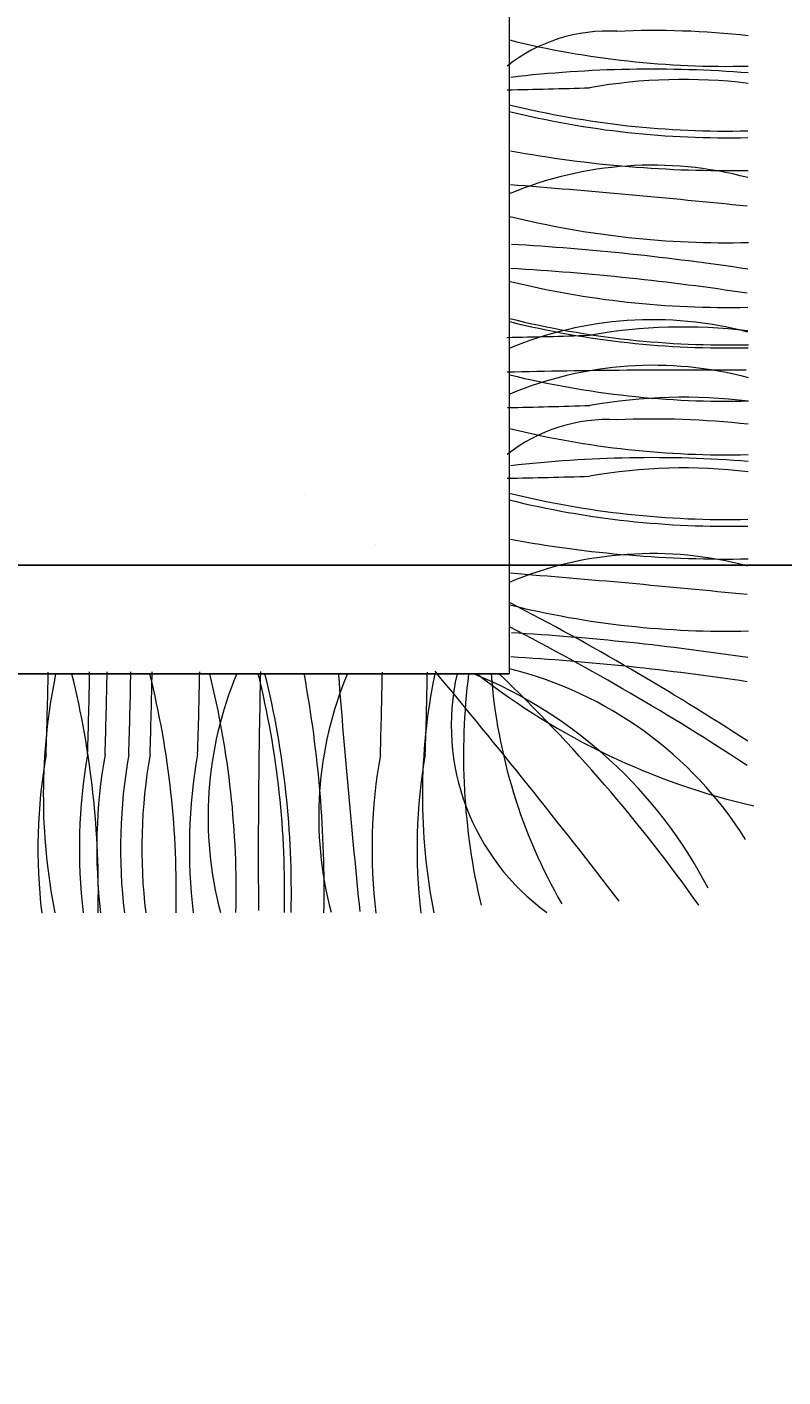
# Model space of a CAD drawing. Units: inches. Extents: x 182 to 1022, y -617 to 111.
# Tile 11 of 33: x 381 to 399, y -308 to -276. Entities that reach past the tile are written whole.
import ezdxf

# ---------------------------------------------------------------- set-up
doc = ezdxf.new("R2010")
doc.units = ezdxf.units.IN
doc.header["$MEASUREMENT"] = 0
doc.layers.add('A-ANNO-DIMS', color=2, linetype='Continuous', lineweight=18)
doc.layers.add('furniture', color=50, linetype='Continuous', lineweight=15, transparency=0.8)
doc.styles.get("Standard").update_dxf_attribs({"font": 'arial.ttf'})
doc.dimstyles.get("Standard").update_dxf_attribs({"dimtxt": 0.18, "dimasz": 0.18, "dimexe": 0.18, "dimexo": 0.0625, "dimgap": 0.09, "dimtad": 0, "dimtih": 1, "dimtoh": 1, "dimdec": 1, "dimzin": 0, "dimdsep": 46, "dimlunit": 4, "dimtxsty": 'Standard', "dimcen": 0.09, "dimadec": 0, "dimazin": 0, "dimtfac": 1, "dimtdec": 1, "dimtofl": 0, "dimtmove": 0, "dimatfit": 3, "dimfxl": 1, "dimtolj": 1, "dimtzin": 0, "dimarcsym": 0})

# ---------------------------------------------------------------- blocks, each defined once
blk = doc.blocks.new('LOUNGE-SEATING-GROUP')
for p, q in [((134.145, 31.682), (134.145, 5.694)), ((137.17, 14.194), (137.17, 14.194)), ((137.705, 14.15), (137.705, 14.15)), ((129.27, 9.969), (129.27, 9.969)), ((130.964, 8.763), (130.964, 8.763)), ((134.145, 5.694), (21.664, 5.694)), ((39.442, 5.694), (134.145, 5.694)), ((130.995, 4.253), (130.995, 4.253)), ((130.995, 4.253), (130.995, 4.253)), ((130.995, 4.253), (130.995, 4.253)), ((132.356, 3.919), (132.356, 3.919)), ((132.356, 3.919), (132.356, 3.919)), ((132.356, 3.919), (132.356, 3.919))]:
    blk.add_line(p, q)
for centre, radius, start, end in [((136.489, 17.128), 3.854, 86.8256, 128.3436), ((137.592, 1.053), 19.942, 83.5587, 92.5565), ((139.313, 41.697), 21.554, 256.1427, 271.3669), ((137.543, -9.04), 29.116, 85.4936, 96.6298), ((131.547, 162.277), 142.714, 271.02248, 271.81091), ((138.293, 7.037), 12.794, 83.1171, 100.0651), ((139.308, 40.158), 21.554, 256.1427, 271.3669), ((139.307, 39.998), 21.554, 256.1427, 271.3669), ((139.339, 46.284), 28.62, 259.5961, 270.9805), ((137.55, 8.956), 8.837, 75.1387, 112.6902), ((114.367, -233.49), 251.596, 84.19829, 85.48538), ((139.318, 37.501), 21.554, 256.1427, 271.3669), ((130.58, -45.595), 61.61, 81.37714, 86.63558), ((130.566, -46.168), 61.61, 81.37714, 86.63558), ((139.301, 35.962), 21.554, 256.1427, 271.3669), ((139.321, 35.071), 21.554, 256.1427, 271.3669), ((137.554, 5.279), 8.837, 75.1387, 112.6902), ((139.309, 34.999), 21.554, 256.1427, 271.3669), ((138.287, 1.148), 12.794, 83.1171, 100.0651), ((131.541, 156.388), 142.714, 271.02248, 271.81091), ((138.51, -171.601), 184.521, 89.60659, 91.37204), ((137.568, 4.195), 8.837, 75.1387, 112.6902), ((139.323, 33.732), 21.554, 256.1427, 271.3669), ((138.299, -0.521), 12.794, 83.1171, 100.0651), ((131.553, 154.719), 142.714, 271.02248, 271.81091), ((136.489, 7.888), 3.854, 86.8256, 128.3436), ((137.592, -8.187), 19.942, 83.5587, 92.5565), ((139.313, 32.457), 21.554, 256.1427, 271.3669), ((137.543, -18.28), 29.116, 85.4936, 96.6298), ((131.547, 153.037), 142.714, 271.02248, 271.81091), ((138.293, -2.203), 12.794, 83.1171, 100.0651), ((139.308, 30.919), 21.554, 256.1427, 271.3669), ((139.307, 30.758), 21.554, 256.1427, 271.3669), ((139.339, 37.044), 28.62, 259.5961, 270.9805), ((137.55, -0.283), 8.837, 75.1387, 112.6902), ((114.367, -242.73), 251.596, 84.19829, 85.48538), ((139.318, 28.261), 21.554, 256.1427, 271.3669), ((105.102, -49.004), 63.435, 56.82194, 62.73315), ((105.088, -49.577), 63.435, 56.82194, 62.73315), ((130.58, -54.835), 61.61, 81.37714, 86.63558), ((131.901, -3.21), 9.302, 32.2712, 76.0065), ((130.566, -55.408), 61.61, 81.37714, 86.63558), ((137.395, 2.803), 14.333, 168.4112, 191.2455), ((-19.513, 8.282), 142.714, 358.18909, 358.97752), ((102.817, 0.521), 21.554, 358.6331, 13.8573), ((-18.527, 8.285), 142.714, 358.18909, 358.97752), ((-18.112, 8.286), 142.714, 358.18909, 358.97752), ((-17.547, 8.287), 142.714, 358.18909, 358.97752), ((104.671, 0.526), 21.554, 358.6331, 13.8573), ((-17.041, 8.289), 142.714, 358.18909, 358.97752), ((-15.91, 8.292), 142.714, 358.18909, 358.97752), ((135.817, 2.285), 8.837, 157.3098, 194.8613), ((106.096, 0.53), 21.554, 358.6331, 13.8573), ((107.248, 0.531), 21.554, 358.6331, 13.8573), ((312.696, 1.329), 184.521, 178.62796, 180.39341), ((107.408, 0.532), 21.554, 358.6331, 13.8573), ((101.122, 0.5), 28.62, 359.0195, 10.4039), ((138.45, 2.289), 8.837, 157.3098, 194.8613), ((380.897, 25.472), 251.596, 184.51462, 185.80171), ((-11.564, 8.279), 142.714, 358.18909, 358.97752), ((146.412, 2.803), 14.333, 168.4112, 191.2455), ((-10.495, 8.282), 142.714, 358.18909, 358.97752), ((-1.664, -106.099), 174.582, 37.54408, 39.84318), ((138.27, 4.474), 5.505, 167.1946, 234.0943), ((148.602, 3.76), 15.545, 172.8509, 193.2785), ((129.187, -4.403), 10.899, 27.3033, 67.8819), ((143.715, 18.887), 16.759, 231.9231, 257.0477), ((146.596, 6.657), 12.919, 184.2757, 209.865), ((107.632, -21.784), 38.017, 35.3153, 46.284), ((135.727, 1.536), 12.794, 169.9349, 186.8829), ((136.713, 1.539), 12.794, 169.9349, 186.8829), ((137.128, 1.54), 12.794, 169.9349, 186.8829), ((137.693, 1.542), 12.794, 169.9349, 186.8829), ((138.199, 1.543), 12.794, 169.9349, 186.8829), ((139.33, 1.546), 12.794, 169.9349, 186.8829), ((143.676, 1.534), 12.794, 169.9349, 186.8829), ((144.745, 1.536), 12.794, 169.9349, 186.8829)]:
    blk.add_arc(centre, radius, start, end)
blk = doc.blocks.new('*D26')
at = {"layer": 'A-ANNO-DIMS', "color": 0, "lineweight": -2, "transparency": 16777216}
for p, q in [((257.848, -296.884), (257.848, -319.733)), ((409.388, -296.884), (409.388, -319.733)), ((258.028, -319.553), (331.642, -319.553)), ((409.208, -319.553), (335.594, -319.553))]:
    blk.add_line(p, q, dxfattribs=at)
at = {"layer": 'A-ANNO-DIMS', "color": 0, "transparency": 16777216}
for points in [[(258.028, -319.523), (258.028, -319.583), (257.848, -319.553)], [(409.208, -319.523), (409.208, -319.583), (409.388, -319.553)]]:
    blk.add_solid(points, dxfattribs=at)
at = {"layer": 'Defpoints', "color": 0, "transparency": 16777216}
for p in [(257.848, -296.822), (409.388, -296.822), (409.388, -319.553)]:
    blk.add_point(p, dxfattribs=at)
at = {"layer": 'A-ANNO-DIMS', "color": 0, "transparency": 16777216, "insert": (333.618, -319.553), "char_height": 0.18, "attachment_point": 5}
blk.add_mtext('\\A1;LOUNGE GROUP 12\'-7 1/2" TYP.', dxfattribs=at)
blk = doc.blocks.new('*D39')
at = {"layer": 'A-ANNO-DIMS', "color": 0, "lineweight": -2, "transparency": 16777216}
for p, q in [((238.398, -288.54), (1015.285, -288.54)), ((1015.105, -288.72), (1015.105, -346.775)), ((1015.105, -405.193), (1015.105, -347.138)), ((238.427, -405.373), (1015.285, -405.373))]:
    blk.add_line(p, q, dxfattribs=at)
at = {"layer": 'A-ANNO-DIMS', "color": 0, "transparency": 16777216}
for points in [[(1015.075, -288.72), (1015.135, -288.72), (1015.105, -288.54)], [(1015.075, -405.193), (1015.135, -405.193), (1015.105, -405.373)]]:
    blk.add_solid(points, dxfattribs=at)
at = {"layer": 'Defpoints', "color": 0, "transparency": 16777216}
for p in [(238.335, -288.54), (1015.105, -288.54), (238.364, -405.373)]:
    blk.add_point(p, dxfattribs=at)
at = {"layer": 'A-ANNO-DIMS', "color": 0, "transparency": 16777216, "insert": (1015.105, -346.956), "char_height": 0.18, "attachment_point": 5}
blk.add_mtext('\\A1;9\'-9"', dxfattribs=at)

msp = doc.modelspace()

# ---------------------------------------------------------------- block references
at = {"layer": 'furniture'}
msp.add_blockref('LOUNGE-SEATING-GROUP', (257.848, -296.822), dxfattribs=at)

# ---------------------------------------------------------------- dimensions: what is measured, and where the dimension line sits
at = {"layer": 'A-ANNO-DIMS'}
dim = msp.add_linear_dim(base=(1015.105, -288.54), p1=(238.364, -405.373), p2=(238.335, -288.54), angle=90, dimstyle='Standard', override={"dimdec": 1, "dimlfac": 1, "dimrnd": 0, "dimzin": 1, "dimdsep": 46, "dimlunit": 4, "dimfrac": 2}, dxfattribs=at)
dim.commit()
dim.dimension.update_dxf_attribs({"geometry": '*D39', "text_midpoint": (1015.105, -346.956)})
dim = msp.add_linear_dim(base=(409.388, -319.553), p1=(257.848, -296.822), p2=(409.388, -296.822), text='LOUNGE GROUP <> TYP.', dimstyle='Standard', override={"dimdec": 1, "dimlfac": 1, "dimrnd": 0, "dimzin": 1, "dimdsep": 46, "dimlunit": 4, "dimfrac": 2}, dxfattribs=at)
dim.commit()
dim.dimension.update_dxf_attribs({"geometry": '*D26', "text_midpoint": (333.618, -319.553)})

doc.saveas('drawing.dxf')
